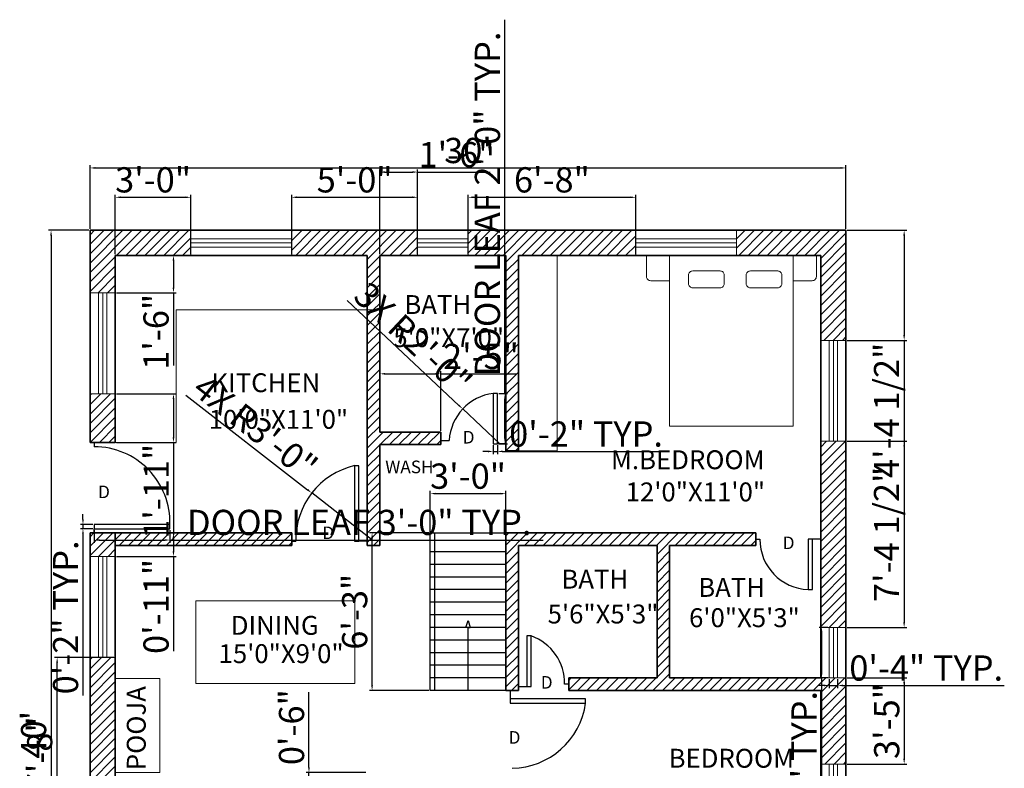
# Model space of a CAD drawing. Units: inches. Extents: x 2105 to 2639, y 1718 to 2373.
# Tile 2 of 2: x 2134 to 2603, y 2017 to 2373. Entities that reach past the tile are written whole.
import ezdxf

# ---------------------------------------------------------------- set-up
doc = ezdxf.new("R2010")
doc.units = ezdxf.units.IN
for name, color, linetype, lineweight in [('A-ANNO-DIMS', 2, 'Continuous', 18), ('A-ANNO-TEXT', 7, 'Continuous', 18), ('A-AREA-IDEN', 7, 'Continuous', 18), ('A-DOOR', 3, 'Continuous', 25), ('A-FLOR-CASE', 9, 'Continuous', 18), ('A-FLOR-STRS', 7, 'Continuous', 25), ('A-FURN', 8, 'Continuous', 18), ('A-GLAZ', 4, 'Continuous', 18), ('A-WALL', 120, 'Continuous', 35), ('A-WALL-PATT', 120, 'Continuous', 13)]:
    doc.layers.add(name, color=color, linetype=linetype, lineweight=lineweight)
doc.styles.get("Standard").update_dxf_attribs({"font": 'arial.ttf'})
doc.dimstyles.new('ISO-25', dxfattribs={"dimtxt": 12, "dimasz": 2.5, "dimexe": 1.25, "dimexo": 0.625, "dimtad": 1, "dimdec": 0, "dimlunit": 3, "dimtxsty": 'Standard', "dimcen": 2.5, "dimadec": 0, "dimazin": 0, "dimtfac": 1, "dimtdec": 0, "dimtmove": 0, "dimatfit": 3, "dimfxl": 1, "dimarcsym": 0})

# ---------------------------------------------------------------- blocks, each defined once
blk = doc.blocks.new('*D1')
at = {"layer": 'A-ANNO-DIMS', "color": 0, "lineweight": -2, "transparency": 16777216}
for p, q in [((2167.87, 2273.92), (2167.87, 2304.21)), ((2170.37, 2302.96), (2525.37, 2302.96)), ((2527.87, 2273.92), (2527.87, 2304.21))]:
    blk.add_line(p, q, dxfattribs=at)
at = {"layer": 'A-ANNO-DIMS', "color": 0, "transparency": 16777216}
for points in [[(2170.37, 2303.38), (2170.37, 2302.54), (2167.87, 2302.96)], [(2525.37, 2303.38), (2525.37, 2302.54), (2527.87, 2302.96)]]:
    blk.add_solid(points, dxfattribs=at)
at = {"layer": 'Defpoints', "color": 0, "transparency": 16777216}
for p in [(2527.87, 2302.96), (2167.87, 2273.29), (2527.87, 2273.29)]:
    blk.add_point(p, dxfattribs=at)
at = {"layer": 'A-ANNO-DIMS', "color": 0, "transparency": 16777216, "insert": (2347.87, 2309.71), "char_height": 12, "attachment_point": 5}
blk.add_mtext("30'", dxfattribs=at)
blk = doc.blocks.new('*D2')
at = {"layer": 'A-ANNO-DIMS', "color": 0, "lineweight": -2, "transparency": 16777216}
for p, q in [((2167.25, 2273.29), (2148.02, 2273.29)), ((2149.27, 2270.79), (2149.27, 1795.79)), ((2167.25, 1793.29), (2148.02, 1793.29))]:
    blk.add_line(p, q, dxfattribs=at)
at = {"layer": 'A-ANNO-DIMS', "color": 0, "transparency": 16777216}
for points in [[(2148.85, 2270.79), (2149.68, 2270.79), (2149.27, 2273.29)], [(2148.85, 1795.79), (2149.68, 1795.79), (2149.27, 1793.29)]]:
    blk.add_solid(points, dxfattribs=at)
at = {"layer": 'Defpoints', "color": 0, "transparency": 16777216}
for p in [(2167.87, 2273.29), (2149.27, 1793.29), (2167.87, 1793.29)]:
    blk.add_point(p, dxfattribs=at)
at = {"layer": 'A-ANNO-DIMS', "color": 0, "transparency": 16777216, "insert": (2142.52, 2033.29), "char_height": 12, "attachment_point": 5, "rotation": 90}
blk.add_mtext("40'", dxfattribs=at)
blk = doc.blocks.new('WIN-GLAZ-48IN')
for p, q in [((0, 4), (48, 4)), ((0, 2), (48, 2)), ((0, 0), (48, 0))]:
    blk.add_line(p, q)
blk = doc.blocks.new('WIN-GLAZ-24IN')
for p, q in [((0, 4), (24, 4)), ((0, 2), (24, 2)), ((0, 0), (24, 0))]:
    blk.add_line(p, q)
blk = doc.blocks.new('DOOR-LEAF-36IN')
for p, q in [((2, 36), (0, 36)), ((0, 36), (0, 0)), ((2, 0), (2, 36)), ((0, 0), (2, 0))]:
    blk.add_line(p, q)
blk = doc.blocks.new('DOOR-LEAF-24IN')
for p, q in [((2, 24), (0, 24)), ((0, 24), (0, 0)), ((2, 0), (2, 24)), ((0, 0), (2, 0))]:
    blk.add_line(p, q)
blk = doc.blocks.new('*D10')
at = {"layer": 'A-ANNO-DIMS', "color": 0, "lineweight": -2, "transparency": 16777216}
for p, q in [((2519.25, 2084.29), (2515.02, 2084.29)), ((2516.27, 2081.79), (2516.27, 2062.79)), ((2519.25, 2060.29), (2515.02, 2060.29)), ((2516.27, 2060.29), (2516.27, 1904.69))]:
    blk.add_line(p, q, dxfattribs=at)
at = {"layer": 'A-ANNO-DIMS', "color": 0, "transparency": 16777216}
for points in [[(2515.86, 2081.79), (2516.69, 2081.79), (2516.27, 2084.29)], [(2515.86, 2062.79), (2516.69, 2062.79), (2516.27, 2060.29)]]:
    blk.add_solid(points, dxfattribs=at)
at = {"layer": 'Defpoints', "color": 0, "transparency": 16777216}
for p in [(2519.87, 2084.29), (2516.27, 2060.29), (2519.87, 2060.29)]:
    blk.add_point(p, dxfattribs=at)
at = {"layer": 'A-ANNO-DIMS', "color": 0, "transparency": 16777216, "insert": (2509.44, 1981.24), "char_height": 12, "attachment_point": 5, "rotation": 90}
blk.add_mtext('WINDOW 2\'-0" TYP.', dxfattribs=at)
blk = doc.blocks.new('*D11')
at = {"layer": 'A-ANNO-DIMS', "color": 0, "lineweight": -2, "transparency": 16777216}
for p, q in [((2519.87, 2059.67), (2519.87, 2055.44)), ((2523.87, 2059.67), (2523.87, 2055.44)), ((2517.37, 2056.69), (2514.87, 2056.69)), ((2519.87, 2056.69), (2523.87, 2056.69)), ((2526.37, 2056.69), (2603.27, 2056.69))]:
    blk.add_line(p, q, dxfattribs=at)
at = {"layer": 'A-ANNO-DIMS', "color": 0, "transparency": 16777216}
for points in [[(2517.37, 2057.11), (2517.37, 2056.28), (2519.87, 2056.69)], [(2526.37, 2057.11), (2526.37, 2056.28), (2523.87, 2056.69)]]:
    blk.add_solid(points, dxfattribs=at)
at = {"layer": 'Defpoints', "color": 0, "transparency": 16777216}
for p in [(2519.87, 2060.29), (2523.87, 2060.29), (2523.87, 2056.69)]:
    blk.add_point(p, dxfattribs=at)
at = {"layer": 'A-ANNO-DIMS', "color": 0, "transparency": 16777216, "insert": (2566.07, 2063.44), "char_height": 12, "attachment_point": 5}
blk.add_mtext('0\'-4" TYP.', dxfattribs=at)
blk = doc.blocks.new('*D12')
at = {"layer": 'A-ANNO-DIMS', "color": 0, "lineweight": -2, "transparency": 16777216}
for p, q in [((2169.87, 2130.67), (2169.87, 2124.64)), ((2205.87, 2130.67), (2205.87, 2124.64)), ((2172.37, 2125.89), (2203.37, 2125.89)), ((2205.87, 2125.89), (2383.71, 2125.89))]:
    blk.add_line(p, q, dxfattribs=at)
at = {"layer": 'A-ANNO-DIMS', "color": 0, "transparency": 16777216}
for points in [[(2172.37, 2126.31), (2172.37, 2125.48), (2169.87, 2125.89)], [(2203.37, 2126.31), (2203.37, 2125.48), (2205.87, 2125.89)]]:
    blk.add_solid(points, dxfattribs=at)
at = {"layer": 'Defpoints', "color": 0, "transparency": 16777216}
for p in [(2169.87, 2131.29), (2205.87, 2131.29), (2205.87, 2125.89)]:
    blk.add_point(p, dxfattribs=at)
at = {"layer": 'A-ANNO-DIMS', "color": 0, "transparency": 16777216, "insert": (2296.04, 2132.73), "char_height": 12, "attachment_point": 5}
blk.add_mtext('DOOR LEAF 3\'-0" TYP.', dxfattribs=at)
blk = doc.blocks.new('*D13')
at = {"layer": 'A-ANNO-DIMS', "color": 0, "lineweight": -2, "transparency": 16777216}
for p, q in [((2164.47, 2135.79), (2164.47, 2138.29)), ((2169.25, 2133.29), (2163.22, 2133.29)), ((2169.25, 2131.29), (2163.22, 2131.29)), ((2164.47, 2133.29), (2164.47, 2131.29)), ((2164.47, 2128.79), (2164.47, 2051.9))]:
    blk.add_line(p, q, dxfattribs=at)
at = {"layer": 'A-ANNO-DIMS', "color": 0, "transparency": 16777216}
for points in [[(2164.06, 2135.79), (2164.89, 2135.79), (2164.47, 2133.29)], [(2164.06, 2128.79), (2164.89, 2128.79), (2164.47, 2131.29)]]:
    blk.add_solid(points, dxfattribs=at)
at = {"layer": 'Defpoints', "color": 0, "transparency": 16777216}
for p in [(2164.47, 2131.29), (2169.87, 2133.29), (2169.87, 2131.29)]:
    blk.add_point(p, dxfattribs=at)
at = {"layer": 'A-ANNO-DIMS', "color": 0, "transparency": 16777216, "insert": (2157.72, 2089.09), "char_height": 12, "attachment_point": 5, "rotation": 90}
blk.add_mtext('0\'-2" TYP.', dxfattribs=at)
blk = doc.blocks.new('*D14')
at = {"layer": 'A-ANNO-DIMS', "color": 0, "lineweight": -2, "transparency": 16777216}
for p, q in [((2365.47, 2195.66), (2365.47, 2373.5)), ((2362.5, 2195.66), (2366.72, 2195.66)), ((2365.47, 2174.16), (2365.47, 2193.16)), ((2362.5, 2171.66), (2366.72, 2171.66))]:
    blk.add_line(p, q, dxfattribs=at)
at = {"layer": 'A-ANNO-DIMS', "color": 0, "transparency": 16777216}
for points in [[(2365.06, 2193.16), (2365.89, 2193.16), (2365.47, 2195.66)], [(2365.06, 2174.16), (2365.89, 2174.16), (2365.47, 2171.66)]]:
    blk.add_solid(points, dxfattribs=at)
at = {"layer": 'Defpoints', "color": 0, "transparency": 16777216}
for p in [(2361.87, 2195.66), (2365.47, 2195.66), (2361.87, 2171.66)]:
    blk.add_point(p, dxfattribs=at)
at = {"layer": 'A-ANNO-DIMS', "color": 0, "transparency": 16777216, "insert": (2358.64, 2285.83), "char_height": 12, "attachment_point": 5, "rotation": 90}
blk.add_mtext('DOOR LEAF 2\'-0" TYP.', dxfattribs=at)
blk = doc.blocks.new('*D15')
at = {"layer": 'A-ANNO-DIMS', "color": 0, "lineweight": -2, "transparency": 16777216}
for p, q in [((2357.37, 2168.06), (2354.87, 2168.06)), ((2359.87, 2171.04), (2359.87, 2166.81)), ((2359.87, 2168.06), (2361.87, 2168.06)), ((2361.87, 2171.04), (2361.87, 2166.81)), ((2364.37, 2168.06), (2441.27, 2168.06))]:
    blk.add_line(p, q, dxfattribs=at)
at = {"layer": 'A-ANNO-DIMS', "color": 0, "transparency": 16777216}
for points in [[(2357.37, 2168.48), (2357.37, 2167.65), (2359.87, 2168.06)], [(2364.37, 2168.48), (2364.37, 2167.65), (2361.87, 2168.06)]]:
    blk.add_solid(points, dxfattribs=at)
at = {"layer": 'Defpoints', "color": 0, "transparency": 16777216}
for p in [(2359.87, 2171.66), (2361.87, 2171.66), (2361.87, 2168.06)]:
    blk.add_point(p, dxfattribs=at)
at = {"layer": 'A-ANNO-DIMS', "color": 0, "transparency": 16777216, "insert": (2404.07, 2174.82), "char_height": 12, "attachment_point": 5}
blk.add_mtext('0\'-2" TYP.', dxfattribs=at)
blk = doc.blocks.new('*D20')
at = {"layer": 'A-ANNO-DIMS', "color": 0, "lineweight": -2, "transparency": 16777216}
for p, q in [((2179.87, 2261.92), (2179.87, 2290.24)), ((2182.37, 2288.99), (2213.37, 2288.99)), ((2215.87, 2261.92), (2215.87, 2290.24))]:
    blk.add_line(p, q, dxfattribs=at)
at = {"layer": 'A-ANNO-DIMS', "color": 0, "transparency": 16777216}
for points in [[(2182.37, 2289.41), (2182.37, 2288.58), (2179.87, 2288.99)], [(2213.37, 2289.41), (2213.37, 2288.58), (2215.87, 2288.99)]]:
    blk.add_solid(points, dxfattribs=at)
at = {"layer": 'Defpoints', "color": 0, "transparency": 16777216}
for p in [(2215.87, 2288.99), (2179.87, 2261.29), (2215.87, 2261.29)]:
    blk.add_point(p, dxfattribs=at)
at = {"layer": 'A-ANNO-DIMS', "color": 0, "transparency": 16777216, "insert": (2197.87, 2295.75), "char_height": 12, "attachment_point": 5}
blk.add_mtext('3\'-0"', dxfattribs=at)
blk = doc.blocks.new('*D21')
at = {"layer": 'A-ANNO-DIMS', "color": 0, "lineweight": -2, "transparency": 16777216}
for p, q in [((2263.87, 2261.92), (2263.87, 2290.24)), ((2266.37, 2288.99), (2321.37, 2288.99)), ((2323.87, 2261.92), (2323.87, 2290.24))]:
    blk.add_line(p, q, dxfattribs=at)
at = {"layer": 'A-ANNO-DIMS', "color": 0, "transparency": 16777216}
for points in [[(2266.37, 2289.41), (2266.37, 2288.58), (2263.87, 2288.99)], [(2321.37, 2289.41), (2321.37, 2288.58), (2323.87, 2288.99)]]:
    blk.add_solid(points, dxfattribs=at)
at = {"layer": 'Defpoints', "color": 0, "transparency": 16777216}
for p in [(2323.87, 2288.99), (2263.87, 2261.29), (2323.87, 2261.29)]:
    blk.add_point(p, dxfattribs=at)
at = {"layer": 'A-ANNO-DIMS', "color": 0, "transparency": 16777216, "insert": (2293.87, 2295.74), "char_height": 12, "attachment_point": 5}
blk.add_mtext('5\'-0"', dxfattribs=at)
blk = doc.blocks.new('*D22')
at = {"layer": 'A-ANNO-DIMS', "color": 0, "lineweight": -2, "transparency": 16777216}
for p, q in [((2347.87, 2261.92), (2347.87, 2290.24)), ((2350.37, 2288.99), (2425.27, 2288.99)), ((2427.77, 2261.92), (2427.77, 2290.24))]:
    blk.add_line(p, q, dxfattribs=at)
at = {"layer": 'A-ANNO-DIMS', "color": 0, "transparency": 16777216}
for points in [[(2350.37, 2289.41), (2350.37, 2288.58), (2347.87, 2288.99)], [(2425.27, 2289.41), (2425.27, 2288.58), (2427.77, 2288.99)]]:
    blk.add_solid(points, dxfattribs=at)
at = {"layer": 'Defpoints', "color": 0, "transparency": 16777216}
for p in [(2427.77, 2288.99), (2347.87, 2261.29), (2427.77, 2261.29)]:
    blk.add_point(p, dxfattribs=at)
at = {"layer": 'A-ANNO-DIMS', "color": 0, "transparency": 16777216, "insert": (2387.82, 2295.74), "char_height": 12, "attachment_point": 5}
blk.add_mtext('6\'-8"', dxfattribs=at)
blk = doc.blocks.new('*D23')
at = {"layer": 'A-ANNO-DIMS', "color": 0, "lineweight": -2, "transparency": 16777216}
for p, q in [((2528.5, 2273.29), (2556.82, 2273.29)), ((2555.57, 2270.79), (2555.57, 2223.42)), ((2528.5, 2220.92), (2556.82, 2220.92)), ((2555.57, 2220.92), (2555.57, 2156.83))]:
    blk.add_line(p, q, dxfattribs=at)
at = {"layer": 'A-ANNO-DIMS', "color": 0, "transparency": 16777216}
for points in [[(2555.16, 2270.79), (2555.99, 2270.79), (2555.57, 2273.29)], [(2555.16, 2223.42), (2555.99, 2223.42), (2555.57, 2220.92)]]:
    blk.add_solid(points, dxfattribs=at)
at = {"layer": 'Defpoints', "color": 0, "transparency": 16777216}
for p in [(2527.87, 2273.29), (2527.87, 2220.92), (2555.57, 2220.92)]:
    blk.add_point(p, dxfattribs=at)
at = {"layer": 'A-ANNO-DIMS', "color": 0, "transparency": 16777216, "insert": (2548.74, 2187.62), "char_height": 12, "attachment_point": 5, "rotation": 90}
blk.add_mtext('4\'-4 1/2"', dxfattribs=at)
blk = doc.blocks.new('*D24')
at = {"layer": 'A-ANNO-DIMS', "color": 0, "lineweight": -2, "transparency": 16777216}
for p, q in [((2528.5, 2172.92), (2556.82, 2172.92)), ((2555.57, 2170.42), (2555.57, 2086.79)), ((2528.5, 2084.29), (2556.82, 2084.29))]:
    blk.add_line(p, q, dxfattribs=at)
at = {"layer": 'A-ANNO-DIMS', "color": 0, "transparency": 16777216}
for points in [[(2555.16, 2170.42), (2555.99, 2170.42), (2555.57, 2172.92)], [(2555.16, 2086.79), (2555.99, 2086.79), (2555.57, 2084.29)]]:
    blk.add_solid(points, dxfattribs=at)
at = {"layer": 'Defpoints', "color": 0, "transparency": 16777216}
for p in [(2527.87, 2172.92), (2527.87, 2084.29), (2555.57, 2084.29)]:
    blk.add_point(p, dxfattribs=at)
at = {"layer": 'A-ANNO-DIMS', "color": 0, "transparency": 16777216, "insert": (2548.74, 2128.61), "char_height": 12, "attachment_point": 5, "rotation": 90}
blk.add_mtext('7\'-4 1/2"', dxfattribs=at)
blk = doc.blocks.new('*D25')
at = {"layer": 'A-ANNO-DIMS', "color": 0, "lineweight": -2, "transparency": 16777216}
for p, q in [((2528.5, 2060.29), (2556.82, 2060.29)), ((2555.57, 2057.79), (2555.57, 2021.81)), ((2528.5, 2019.31), (2556.82, 2019.31))]:
    blk.add_line(p, q, dxfattribs=at)
at = {"layer": 'A-ANNO-DIMS', "color": 0, "transparency": 16777216}
for points in [[(2555.16, 2057.79), (2555.99, 2057.79), (2555.57, 2060.29)], [(2555.16, 2021.81), (2555.99, 2021.81), (2555.57, 2019.31)]]:
    blk.add_solid(points, dxfattribs=at)
at = {"layer": 'Defpoints', "color": 0, "transparency": 16777216}
for p in [(2527.87, 2060.29), (2527.87, 2019.31), (2555.57, 2019.31)]:
    blk.add_point(p, dxfattribs=at)
at = {"layer": 'A-ANNO-DIMS', "color": 0, "transparency": 16777216, "insert": (2548.82, 2039.8), "char_height": 12, "attachment_point": 5, "rotation": 90}
blk.add_mtext('3\'-5"', dxfattribs=at)
blk = doc.blocks.new('*D28')
at = {"layer": 'A-ANNO-DIMS', "color": 0, "lineweight": -2, "transparency": 16777216}
for p, q in [((2180.5, 2261.29), (2208.82, 2261.29)), ((2207.57, 2258.79), (2207.57, 2246.01)), ((2180.5, 2243.51), (2208.82, 2243.51)), ((2207.57, 2243.51), (2207.57, 2208.99))]:
    blk.add_line(p, q, dxfattribs=at)
at = {"layer": 'A-ANNO-DIMS', "color": 0, "transparency": 16777216}
for points in [[(2207.16, 2258.79), (2207.99, 2258.79), (2207.57, 2261.29)], [(2207.16, 2246.01), (2207.99, 2246.01), (2207.57, 2243.51)]]:
    blk.add_solid(points, dxfattribs=at)
at = {"layer": 'Defpoints', "color": 0, "transparency": 16777216}
for p in [(2179.87, 2261.29), (2179.87, 2243.51), (2207.57, 2243.51)]:
    blk.add_point(p, dxfattribs=at)
at = {"layer": 'A-ANNO-DIMS', "color": 0, "transparency": 16777216, "insert": (2200.82, 2225), "char_height": 12, "attachment_point": 5, "rotation": 90}
blk.add_mtext('1\'-6"', dxfattribs=at)
blk = doc.blocks.new('*D29')
at = {"layer": 'A-ANNO-DIMS', "color": 0, "lineweight": -2, "transparency": 16777216}
for p, q in [((2180.5, 2195.51), (2208.82, 2195.51)), ((2207.57, 2193.01), (2207.57, 2174.79)), ((2180.5, 2172.29), (2208.82, 2172.29)), ((2207.57, 2172.29), (2207.57, 2128.45))]:
    blk.add_line(p, q, dxfattribs=at)
at = {"layer": 'A-ANNO-DIMS', "color": 0, "transparency": 16777216}
for points in [[(2207.16, 2193.01), (2207.99, 2193.01), (2207.57, 2195.51)], [(2207.16, 2174.79), (2207.99, 2174.79), (2207.57, 2172.29)]]:
    blk.add_solid(points, dxfattribs=at)
at = {"layer": 'Defpoints', "color": 0, "transparency": 16777216}
for p in [(2179.87, 2195.51), (2179.87, 2172.29), (2207.57, 2172.29)]:
    blk.add_point(p, dxfattribs=at)
at = {"layer": 'A-ANNO-DIMS', "color": 0, "transparency": 16777216, "insert": (2200.92, 2149.12), "char_height": 12, "attachment_point": 5, "rotation": 90}
blk.add_mtext('1\'-11"', dxfattribs=at)
blk = doc.blocks.new('*D30')
at = {"layer": 'A-ANNO-DIMS', "color": 0, "lineweight": -2, "transparency": 16777216}
for p, q in [((2180.5, 2129.29), (2208.82, 2129.29)), ((2207.57, 2126.79), (2207.57, 2120.56)), ((2180.5, 2118.06), (2208.82, 2118.06)), ((2207.57, 2118.06), (2207.57, 2073.09))]:
    blk.add_line(p, q, dxfattribs=at)
at = {"layer": 'A-ANNO-DIMS', "color": 0, "transparency": 16777216}
for points in [[(2207.16, 2126.79), (2207.99, 2126.79), (2207.57, 2129.29)], [(2207.16, 2120.56), (2207.99, 2120.56), (2207.57, 2118.06)]]:
    blk.add_solid(points, dxfattribs=at)
at = {"layer": 'Defpoints', "color": 0, "transparency": 16777216}
for p in [(2179.87, 2129.29), (2179.87, 2118.06), (2207.57, 2118.06)]:
    blk.add_point(p, dxfattribs=at)
at = {"layer": 'A-ANNO-DIMS', "color": 0, "transparency": 16777216, "insert": (2200.82, 2094.32), "char_height": 12, "attachment_point": 5, "rotation": 90}
blk.add_mtext('0\'-11"', dxfattribs=at)
blk = doc.blocks.new('*D31')
at = {"layer": 'A-ANNO-DIMS', "color": 0, "lineweight": -2, "transparency": 16777216}
for p, q in [((2179.25, 2070.06), (2150.92, 2070.06)), ((2152.17, 1980.35), (2152.17, 2067.56)), ((2179.25, 1977.85), (2150.92, 1977.85))]:
    blk.add_line(p, q, dxfattribs=at)
at = {"layer": 'A-ANNO-DIMS', "color": 0, "transparency": 16777216}
for points in [[(2151.76, 2067.56), (2152.59, 2067.56), (2152.17, 2070.06)], [(2151.76, 1980.35), (2152.59, 1980.35), (2152.17, 1977.85)]]:
    blk.add_solid(points, dxfattribs=at)
at = {"layer": 'Defpoints', "color": 0, "transparency": 16777216}
for p in [(2152.17, 2070.06), (2179.87, 2070.06), (2179.87, 1977.85)]:
    blk.add_point(p, dxfattribs=at)
at = {"layer": 'A-ANNO-DIMS', "color": 0, "transparency": 16777216, "insert": (2145.42, 2023.95), "char_height": 12, "attachment_point": 5, "rotation": 90}
blk.add_mtext('7\'-8"', dxfattribs=at)
blk = doc.blocks.new('*D35')
at = {"layer": 'A-ANNO-DIMS', "color": 0, "lineweight": -2, "transparency": 16777216}
for p, q in [((2329.87, 2120.92), (2329.87, 2149.24)), ((2332.37, 2147.99), (2363.37, 2147.99)), ((2365.87, 2120.92), (2365.87, 2149.24))]:
    blk.add_line(p, q, dxfattribs=at)
at = {"layer": 'A-ANNO-DIMS', "color": 0, "transparency": 16777216}
for points in [[(2332.37, 2148.41), (2332.37, 2147.58), (2329.87, 2147.99)], [(2363.37, 2148.41), (2363.37, 2147.58), (2365.87, 2147.99)]]:
    blk.add_solid(points, dxfattribs=at)
at = {"layer": 'Defpoints', "color": 0, "transparency": 16777216}
for p in [(2365.87, 2147.99), (2329.87, 2120.29), (2365.87, 2120.29)]:
    blk.add_point(p, dxfattribs=at)
at = {"layer": 'A-ANNO-DIMS', "color": 0, "transparency": 16777216, "insert": (2347.87, 2154.75), "char_height": 12, "attachment_point": 5}
blk.add_mtext('3\'-0"', dxfattribs=at)
blk = doc.blocks.new('*D36')
at = {"layer": 'A-ANNO-DIMS', "color": 0, "lineweight": -2, "transparency": 16777216}
for p, q in [((2329.25, 2129.29), (2300.92, 2129.29)), ((2302.17, 2056.79), (2302.17, 2126.79)), ((2329.25, 2054.29), (2300.92, 2054.29))]:
    blk.add_line(p, q, dxfattribs=at)
at = {"layer": 'A-ANNO-DIMS', "color": 0, "transparency": 16777216}
for points in [[(2301.76, 2126.79), (2302.59, 2126.79), (2302.17, 2129.29)], [(2301.76, 2056.79), (2302.59, 2056.79), (2302.17, 2054.29)]]:
    blk.add_solid(points, dxfattribs=at)
at = {"layer": 'Defpoints', "color": 0, "transparency": 16777216}
for p in [(2302.17, 2129.29), (2329.87, 2129.29), (2329.87, 2054.29)]:
    blk.add_point(p, dxfattribs=at)
at = {"layer": 'A-ANNO-DIMS', "color": 0, "transparency": 16777216, "insert": (2295.42, 2091.79), "char_height": 12, "attachment_point": 5, "rotation": 90}
blk.add_mtext('6\'-3"', dxfattribs=at)
blk = doc.blocks.new('*D38')
at = {"layer": 'A-ANNO-DIMS', "color": 0, "lineweight": -2, "transparency": 16777216}
for p, q in [((2272.1, 2017.79), (2272.1, 2053.44)), ((2299.18, 2015.29), (2270.85, 2015.29)), ((2272.1, 2009.29), (2272.1, 2015.29)), ((2299.18, 2009.29), (2270.85, 2009.29)), ((2272.1, 2006.79), (2272.1, 2004.29))]:
    blk.add_line(p, q, dxfattribs=at)
at = {"layer": 'A-ANNO-DIMS', "color": 0, "transparency": 16777216}
for points in [[(2271.69, 2017.79), (2272.52, 2017.79), (2272.1, 2015.29)], [(2271.69, 2006.79), (2272.52, 2006.79), (2272.1, 2009.29)]]:
    blk.add_solid(points, dxfattribs=at)
at = {"layer": 'Defpoints', "color": 0, "transparency": 16777216}
for p in [(2272.1, 2015.29), (2299.8, 2015.29), (2299.8, 2009.29)]:
    blk.add_point(p, dxfattribs=at)
at = {"layer": 'A-ANNO-DIMS', "color": 0, "transparency": 16777216, "insert": (2265.35, 2036.87), "char_height": 12, "attachment_point": 5, "rotation": 90}
blk.add_mtext('0\'-6"', dxfattribs=at)
blk = doc.blocks.new('*D39')
at = {"layer": 'A-ANNO-DIMS', "color": 0, "lineweight": -2, "transparency": 16777216}
for p, q in [((2305.87, 2177.92), (2305.87, 2206.24)), ((2308.37, 2204.99), (2332.37, 2204.99)), ((2334.87, 2177.92), (2334.87, 2206.24)), ((2334.87, 2204.99), (2370.73, 2204.99))]:
    blk.add_line(p, q, dxfattribs=at)
at = {"layer": 'A-ANNO-DIMS', "color": 0, "transparency": 16777216}
for points in [[(2308.37, 2205.41), (2308.37, 2204.58), (2305.87, 2204.99)], [(2332.37, 2205.41), (2332.37, 2204.58), (2334.87, 2204.99)]]:
    blk.add_solid(points, dxfattribs=at)
at = {"layer": 'Defpoints', "color": 0, "transparency": 16777216}
for p in [(2334.87, 2204.99), (2305.87, 2177.29), (2334.87, 2177.29)]:
    blk.add_point(p, dxfattribs=at)
at = {"layer": 'A-ANNO-DIMS', "color": 0, "transparency": 16777216, "insert": (2354.05, 2211.74), "char_height": 12, "attachment_point": 5}
blk.add_mtext('2\'-5"', dxfattribs=at)
blk = doc.blocks.new('*D40')
at = {"layer": 'A-ANNO-DIMS', "color": 0, "lineweight": -2, "transparency": 16777216}
for p, q in [((2305.87, 2261.92), (2305.87, 2302.24)), ((2308.37, 2300.99), (2321.37, 2300.99)), ((2323.87, 2261.92), (2323.87, 2302.24)), ((2323.87, 2300.99), (2358.39, 2300.99))]:
    blk.add_line(p, q, dxfattribs=at)
at = {"layer": 'A-ANNO-DIMS', "color": 0, "transparency": 16777216}
for points in [[(2308.37, 2301.41), (2308.37, 2300.58), (2305.87, 2300.99)], [(2321.37, 2301.41), (2321.37, 2300.58), (2323.87, 2300.99)]]:
    blk.add_solid(points, dxfattribs=at)
at = {"layer": 'Defpoints', "color": 0, "transparency": 16777216}
for p in [(2323.87, 2300.99), (2305.87, 2261.29), (2323.87, 2261.29)]:
    blk.add_point(p, dxfattribs=at)
at = {"layer": 'A-ANNO-DIMS', "color": 0, "transparency": 16777216, "insert": (2342.38, 2307.74), "char_height": 12, "attachment_point": 5}
blk.add_mtext('1\'-6"', dxfattribs=at)
blk = doc.blocks.new('*D42')
at = {"layer": 'A-ANNO-DIMS', "color": 0, "lineweight": -2, "transparency": 16777216}
for p, q in [((2213.53, 2194.89), (2271.47, 2149.83)), ((2301.86, 2126.19), (2273.45, 2148.29))]:
    blk.add_line(p, q, dxfattribs=at)
at = {"layer": 'A-ANNO-DIMS', "color": 0, "transparency": 16777216}
blk.add_solid([(2271.73, 2150.15), (2271.22, 2149.5), (2273.45, 2148.29)], dxfattribs=at)
at = {"layer": 'Defpoints', "color": 0, "transparency": 16777216}
for p in [(2273.45, 2148.29), (2301.86, 2126.19)]:
    blk.add_point(p, dxfattribs=at)
at = {"layer": 'A-ANNO-DIMS', "color": 0, "transparency": 16777216, "insert": (2245.66, 2178.46), "char_height": 12, "attachment_point": 5, "rotation": 322.1257}
blk.add_mtext('4X R3\'-0"', dxfattribs=at)
blk = doc.blocks.new('*D43')
at = {"layer": 'A-ANNO-DIMS', "color": 0, "lineweight": -2, "transparency": 16777216}
for p, q in [((2290.35, 2239.88), (2343.51, 2189.98)), ((2362.83, 2171.85), (2345.33, 2188.27))]:
    blk.add_line(p, q, dxfattribs=at)
at = {"layer": 'A-ANNO-DIMS', "color": 0, "transparency": 16777216}
blk.add_solid([(2343.79, 2190.29), (2343.22, 2189.68), (2345.33, 2188.27)], dxfattribs=at)
at = {"layer": 'Defpoints', "color": 0, "transparency": 16777216}
for p in [(2345.33, 2188.27), (2362.83, 2171.85)]:
    blk.add_point(p, dxfattribs=at)
at = {"layer": 'A-ANNO-DIMS', "color": 0, "transparency": 16777216, "insert": (2320.64, 2220.71), "char_height": 12, "attachment_point": 5, "rotation": 316.8117}
blk.add_mtext('3X R2\'-0"', dxfattribs=at)

msp = doc.modelspace()

# ---------------------------------------------------------------- hatches: boundary and pattern name
at = {"layer": 'A-WALL-PATT'}
h = msp.add_hatch(dxfattribs=at)
h.set_pattern_fill('ANSI31', color=256)
h.paths.add_polyline_path([(2215.87, 2273.29), (2167.87, 2273.29), (2167.87, 2243.51), (2179.87, 2243.51), (2179.87, 2261.29), (2215.87, 2261.29)])
h = msp.add_hatch(dxfattribs=at)
h.set_pattern_fill('ANSI31', color=256)
h.paths.add_polyline_path([(2323.87, 2273.29), (2263.87, 2273.29), (2263.87, 2261.29), (2299.87, 2261.29), (2299.87, 2235.4), (2305.87, 2235.4), (2305.87, 2261.29), (2323.87, 2261.29)])
h = msp.add_hatch(dxfattribs=at)
h.set_pattern_fill('ANSI31', color=256)
h.paths.add_polyline_path([(2427.77, 2273.29), (2347.87, 2273.29), (2347.87, 2261.29), (2365.87, 2261.29), (2365.87, 2168.36), (2371.87, 2168.36), (2371.87, 2261.29), (2427.77, 2261.29)])
h = msp.add_hatch(dxfattribs=at)
h.set_pattern_fill('ANSI31', color=256)
h.paths.add_polyline_path([(2527.87, 2273.29), (2475.77, 2273.29), (2475.77, 2261.29), (2502.75, 2261.29), (2515.87, 2261.29), (2515.87, 2220.92), (2527.87, 2220.92)])
h = msp.add_hatch(dxfattribs=at)
h.set_pattern_fill('ANSI31', color=256)
h.paths.add_polyline_path([(2305.87, 2235.4), (2299.87, 2235.4), (2299.87, 2129.29), (2299.87, 2123.29), (2305.87, 2123.29), (2305.87, 2171.29), (2334.87, 2171.29), (2334.87, 2173.29), (2334.87, 2177.29), (2305.87, 2177.29)])
h = msp.add_hatch(dxfattribs=at)
h.set_pattern_fill('ANSI31', color=256)
h.paths.add_polyline_path([(2179.87, 2195.51), (2167.87, 2195.51), (2167.87, 2172.29), (2169.87, 2172.29), (2179.87, 2172.29)])
h = msp.add_hatch(dxfattribs=at)
h.set_pattern_fill('ANSI31', color=256)
h.paths.add_polyline_path([(2527.87, 2172.92), (2515.87, 2172.92), (2515.87, 2084.29), (2527.87, 2084.29)])
h = msp.add_hatch(dxfattribs=at)
h.set_pattern_fill('ANSI31', color=256)
h.paths.add_polyline_path([(2179.87, 2129.29), (2167.87, 2129.29), (2167.87, 2118.06), (2179.87, 2118.06)])
h = msp.add_hatch(dxfattribs=at)
h.set_pattern_fill('ANSI31', color=256)
h.paths.add_polyline_path([(2263.87, 2129.29), (2179.87, 2129.29), (2179.87, 2123.29), (2263.87, 2123.29), (2263.87, 2125.29)])
h = msp.add_hatch(dxfattribs=at)
h.set_pattern_fill('ANSI31', color=256)
h.paths.add_polyline_path([(2527.87, 2060.29), (2515.87, 2060.29), (2443.87, 2060.29), (2443.87, 2123.29), (2484.87, 2123.29), (2484.87, 2129.29), (2365.87, 2129.29), (2365.87, 2054.29), (2367.87, 2054.29), (2371.87, 2054.29), (2371.87, 2056.29), (2371.87, 2123.29), (2437.87, 2123.29), (2437.87, 2060.29), (2395.87, 2060.29), (2395.87, 2054.29), (2515.87, 2054.29), (2515.87, 2019.31), (2527.87, 2019.31)])
h = msp.add_hatch(dxfattribs=at)
h.set_pattern_fill('ANSI31', color=256)
h.paths.add_polyline_path([(2179.87, 2070.06), (2167.87, 2070.06), (2167.87, 1977.85), (2179.87, 1977.85)])

# ---------------------------------------------------------------- linework, layer by layer
at = {"layer": 'A-DOOR'}
for p, q in [((2167.87, 2172.29), (2169.87, 2172.29)), ((2169.87, 2172.29), (2169.87, 2170.29)), ((2334.87, 2171.29), (2334.87, 2173.29)), ((2334.87, 2173.29), (2338.87, 2173.29)), ((2365.87, 2171.66), (2361.87, 2171.66)), ((2365.87, 2168.36), (2365.87, 2171.66)), ((2167.87, 2129.29), (2169.87, 2129.29)), ((2169.87, 2129.29), (2169.87, 2131.29)), ((2484.87, 2129.29), (2484.87, 2126.29)), ((2515.87, 2129.29), (2515.87, 2126.29)), ((2263.87, 2123.29), (2263.87, 2125.29)), ((2263.87, 2125.29), (2265.87, 2125.29)), ((2299.87, 2125.29), (2295.87, 2125.29)), ((2299.87, 2123.29), (2299.87, 2125.29)), ((2484.87, 2126.29), (2486.87, 2126.29)), ((2515.87, 2126.29), (2511.87, 2126.29)), ((2365.87, 2054.29), (2367.87, 2054.29)), ((2367.87, 2054.29), (2367.87, 2050.29)), ((2371.87, 2054.29), (2371.87, 2056.29)), ((2371.87, 2056.29), (2375.87, 2056.29)), ((2395.87, 2057.29), (2393.87, 2057.29)), ((2395.87, 2054.29), (2395.87, 2057.29))]:
    msp.add_line(p, q, dxfattribs=at)
for centre, radius, start, end in [((2362.83, 2171.85), 24, 97.0761, 176.5494), ((2169.89, 2134.29), 36, 358.4082, 90.0221), ((2301.86, 2126.19), 36, 102.8213, 181.4287), ((2510.87, 2126.27), 24, 179.9502, 267.612), ((2369.88, 2057.66), 24, 359.1129, 70.5361), ((2368.22, 2053.29), 36, 271.0376, 352.0259)]:
    msp.add_arc(centre, radius, start, end, dxfattribs=at)
at = {"layer": 'A-FLOR-CASE'}
for p, q in [((2390.24, 2168.36), (2390.24, 2261.29)), ((2208.82, 2172.29), (2208.82, 2235.4)), ((2208.82, 2235.4), (2305.87, 2235.4)), ((2179.87, 2172.29), (2208.82, 2172.29)), ((2371.87, 2168.36), (2390.24, 2168.36))]:
    msp.add_line(p, q, dxfattribs=at)
msp.add_lwpolyline([(2179.87, 2015.29), (2201.1, 2015.29), (2201.1, 2060.06), (2179.87, 2060.06)], close=True, dxfattribs=at)
at = {"layer": 'A-FLOR-STRS'}
for p, q in [((2329.87, 2054.29), (2329.87, 2129.29)), ((2329.87, 2129.29), (2365.87, 2129.29)), ((2329.87, 2129.29), (2331.87, 2129.29)), ((2331.87, 2129.29), (2331.87, 2054.29)), ((2365.87, 2120.29), (2329.87, 2120.29)), ((2365.87, 2120.29), (2329.87, 2120.29)), ((2365.87, 2114.29), (2329.87, 2114.29)), ((2365.87, 2108.29), (2329.87, 2108.29)), ((2365.87, 2102.29), (2329.87, 2102.29)), ((2365.87, 2096.29), (2329.87, 2096.29)), ((2365.87, 2090.29), (2329.87, 2090.29)), ((2346.87, 2084.29), (2347.87, 2087.56)), ((2347.87, 2087.56), (2348.87, 2084.29)), ((2365.87, 2084.29), (2329.87, 2084.29)), ((2347.87, 2084.29), (2346.87, 2084.29)), ((2347.87, 2054.29), (2347.87, 2084.29)), ((2347.87, 2084.29), (2348.87, 2084.29)), ((2365.87, 2078.29), (2329.87, 2078.29)), ((2365.87, 2072.29), (2329.87, 2072.29)), ((2365.87, 2066.29), (2329.87, 2066.29)), ((2365.87, 2060.29), (2329.87, 2060.29)), ((2365.87, 2054.29), (2329.87, 2054.29))]:
    msp.add_line(p, q, dxfattribs=at)
at = {"layer": 'A-FURN'}
for points in [[(2443.87, 2261.29), (2432.87, 2261.29), (2432.87, 2251.29, 0.414214), (2434.87, 2249.29), (2443.87, 2249.29)], [(2502.75, 2261.29), (2513.75, 2261.29), (2513.75, 2251.29, -0.414214), (2511.75, 2249.29), (2502.75, 2249.29)], [(2454.89, 2253.95), (2467.89, 2253.95, -0.414214), (2469.89, 2251.95), (2469.89, 2247.95, -0.414214), (2467.89, 2245.95), (2454.89, 2245.95, -0.414214), (2452.89, 2247.95), (2452.89, 2251.95, -0.414214)], [(2482.33, 2253.95), (2495.33, 2253.95, -0.414214), (2497.33, 2251.95), (2497.33, 2247.95, -0.414214), (2495.33, 2245.95), (2482.33, 2245.95, -0.414214), (2480.33, 2247.95), (2480.33, 2251.95, -0.414214)]]:
    msp.add_lwpolyline(points, format="xyb", close=True, dxfattribs=at)
for points in [[(2443.87, 2261.29), (2502.75, 2261.29), (2502.75, 2180.11), (2443.87, 2180.11)], [(2218.16, 2097), (2294.01, 2097), (2294.01, 2057.69), (2218.16, 2057.69)]]:
    msp.add_lwpolyline(points, close=True, dxfattribs=at)
at = {"layer": 'A-GLAZ'}
for p, q in [((2215.87, 2261.29), (2215.87, 2273.29)), ((2263.87, 2261.29), (2263.87, 2273.29)), ((2323.87, 2261.29), (2323.87, 2273.29)), ((2347.87, 2261.29), (2347.87, 2273.29)), ((2427.77, 2261.29), (2427.77, 2273.29)), ((2475.77, 2261.29), (2475.77, 2273.29)), ((2167.87, 2243.51), (2179.87, 2243.51)), ((2527.87, 2220.92), (2515.87, 2220.92)), ((2167.87, 2195.51), (2179.87, 2195.51)), ((2527.87, 2172.92), (2515.87, 2172.92)), ((2167.87, 2118.06), (2179.87, 2118.06)), ((2527.87, 2084.29), (2515.87, 2084.29)), ((2167.87, 2070.06), (2179.87, 2070.06)), ((2527.87, 2060.29), (2515.87, 2060.29)), ((2527.87, 2019.31), (2515.87, 2019.31))]:
    msp.add_line(p, q, dxfattribs=at)
at = {"layer": 'A-WALL'}
for p, q in [((2179.87, 2261.29), (2299.87, 2261.29)), ((2179.87, 2172.29), (2179.87, 2261.29)), ((2299.87, 2129.29), (2299.87, 2261.29)), ((2305.87, 2177.29), (2305.87, 2261.29)), ((2305.87, 2261.29), (2365.87, 2261.29)), ((2365.87, 2168.36), (2365.87, 2261.29)), ((2371.87, 2168.36), (2371.87, 2261.29)), ((2371.87, 2261.29), (2515.87, 2261.29)), ((2515.87, 2261.29), (2515.87, 2060.29)), ((2305.87, 2177.29), (2334.87, 2177.29)), ((2334.87, 2171.29), (2334.87, 2177.29)), ((2179.87, 2172.29), (2167.87, 2172.29)), ((2305.87, 2123.29), (2305.87, 2171.29)), ((2305.87, 2171.29), (2334.87, 2171.29)), ((2365.87, 2168.36), (2371.87, 2168.36)), ((2179.87, 2129.29), (2167.87, 2129.29)), ((2179.87, 1865.29), (2179.87, 2129.29)), ((2179.87, 2129.29), (2263.87, 2129.29)), ((2263.87, 2129.29), (2263.87, 2123.29)), ((2299.87, 2129.29), (2299.87, 2123.29)), ((2365.87, 2129.29), (2484.87, 2129.29)), ((2365.87, 2054.29), (2365.87, 2129.29)), ((2484.87, 2129.29), (2484.87, 2123.29)), ((2515.87, 2129.29), (2515.87, 2123.29)), ((2179.87, 2123.29), (2263.87, 2123.29)), ((2299.87, 2123.29), (2305.87, 2123.29)), ((2371.87, 2123.29), (2437.87, 2123.29)), ((2371.87, 2054.29), (2371.87, 2123.29)), ((2437.87, 2060.29), (2437.87, 2123.29)), ((2443.87, 2060.29), (2443.87, 2123.29)), ((2443.87, 2123.29), (2484.87, 2123.29)), ((2395.87, 2060.29), (2437.87, 2060.29)), ((2395.87, 2054.29), (2395.87, 2060.29)), ((2443.87, 2060.29), (2515.87, 2060.29)), ((2365.87, 2054.29), (2371.87, 2054.29)), ((2395.87, 2054.29), (2515.87, 2054.29)), ((2515.87, 2054.29), (2515.87, 1931.29))]:
    msp.add_line(p, q, dxfattribs=at)
msp.add_lwpolyline([(2167.87, 2172.29), (2167.87, 2273.29), (2527.87, 2273.29), (2527.87, 1793.29), (2167.87, 1793.29), (2167.87, 2129.29)], dxfattribs=at)

# ---------------------------------------------------------------- block references
at = {"layer": 'A-DOOR'}
for name, p in [('DOOR-LEAF-24IN', (2359.87, 2171.66)), ('DOOR-LEAF-36IN', (2293.87, 2125.29)), ('DOOR-LEAF-24IN', (2509.87, 2102.29))]:
    msp.add_blockref(name, p, dxfattribs=at)
for name, p, rotation in [('DOOR-LEAF-36IN', (2169.87, 2133.29), 269.9999999999942), ('DOOR-LEAF-24IN', (2377.87, 2080.29), 180), ('DOOR-LEAF-36IN', (2403.87, 2048.29), 89.99999999999714)]:
    msp.add_blockref(name, p, dxfattribs=dict(at, rotation=rotation))
at = {"layer": 'A-GLAZ'}
for name, p in [('WIN-GLAZ-48IN', (2215.87, 2265.29)), ('WIN-GLAZ-24IN', (2323.87, 2265.29))]:
    msp.add_blockref(name, p, dxfattribs=at)
for name, p, rotation in [('WIN-GLAZ-48IN', (2475.77, 2269.29), 180), ('WIN-GLAZ-48IN', (2175.87, 2195.51), 90.00000000000097), ('WIN-GLAZ-48IN', (2519.87, 2220.92), 270.0000000000021), ('WIN-GLAZ-48IN', (2175.87, 2070.06), 90.00000000000205), ('WIN-GLAZ-24IN', (2519.87, 2084.29), 269.9999999999961), ('WIN-GLAZ-48IN', (2519.87, 2019.31), 270.0000000000023)]:
    msp.add_blockref(name, p, dxfattribs=dict(at, rotation=rotation))

# ---------------------------------------------------------------- texts
at = {"layer": 'A-ANNO-TEXT'}
for p in [(2345.34, 2171.83), (2171.67, 2145.83), (2278.51, 2126.34), (2497.73, 2121.57), (2382.52, 2055.18), (2367.2, 2028.98)]:
    msp.add_attdef('D', p, '', height=6, dxfattribs=at)
at = {"layer": 'A-AREA-IDEN'}
for tag, p, height in [('BATH', (2317.54, 2233.45), 9), ('5\'0"X7\'0"', (2312.29, 2217.72), 9), ('KITCHEN', (2225.7, 2196.26), 9), ('10\'0"X11\'0"', (2224.38, 2178.83), 9), ('M.BEDROOM', (2415.95, 2159.6), 9), ('WASH', (2308.44, 2157.71), 6), ('12\'0"X11\'0"', (2422.94, 2144.3), 9), ('BATH', (2392.33, 2102.79), 9), ('BATH', (2457.5, 2098.86), 9), ('5\'6"X5\'3"', (2385.77, 2086.19), 9), ('6\'0"X5\'3"', (2453.12, 2084.44), 9), ('DINING', (2234.88, 2080.81), 9), ('15\'0"X9\'0"', (2229.05, 2067.34), 9), ('BEDROOM', (2443.39, 2017.56), 9)]:
    msp.add_attdef(tag, p, '', height=height, dxfattribs=at)
msp.add_attdef('POOJA', (2194.36, 2016.39), '', height=9, rotation=90, dxfattribs=at)

# ---------------------------------------------------------------- dimensions: what is measured, and where the dimension line sits
at = {"layer": 'A-ANNO-DIMS'}
for base, p1, p2, angle, text, picture, middle in [((2365.47, 2195.66), (2361.87, 2171.66), (2361.87, 2195.66), 90, 'DOOR LEAF <> TYP.', '*D14', (2358.64, 2285.83)), ((2164.47, 2131.29), (2169.87, 2133.29), (2169.87, 2131.29), 270, '<> TYP.', '*D13', (2157.72, 2089.09)), ((2516.27, 2060.29), (2519.87, 2084.29), (2519.87, 2060.29), 270, 'WINDOW <> TYP.', '*D10', (2509.44, 1981.24))]:
    dim = msp.add_linear_dim(base=base, p1=p1, p2=p2, angle=angle, text=text, dimstyle='ISO-25', override={"dimdec": 1, "dimlfac": 1, "dimrnd": 0, "dimzin": 1, "dimdsep": 46, "dimlunit": 4, "dimfrac": 2}, dxfattribs=at)
    dim.commit()
    dim.dimension.update_dxf_attribs({"geometry": picture, "text_midpoint": middle})
for base, p1, p2, override, picture, middle in [((2527.87, 2302.96), (2167.87, 2273.29), (2527.87, 2273.29), {"dimclrd": 0, "dimclre": 0, "dimclrt": 0}, '*D1', (2347.87, 2309.71)), ((2323.87, 2300.99), (2305.87, 2261.29), (2323.87, 2261.29), {"dimdec": 1, "dimlfac": 1, "dimrnd": 0, "dimzin": 1, "dimdsep": 46, "dimlunit": 4, "dimfrac": 2}, '*D40', (2342.38, 2307.74)), ((2215.87, 2288.99), (2179.87, 2261.29), (2215.87, 2261.29), {"dimdec": 1, "dimlfac": 1, "dimrnd": 0, "dimzin": 1, "dimdsep": 46, "dimlunit": 4, "dimfrac": 2}, '*D20', (2197.87, 2295.75)), ((2323.87, 2288.99), (2263.87, 2261.29), (2323.87, 2261.29), {"dimdec": 1, "dimlfac": 1, "dimrnd": 0, "dimzin": 1, "dimdsep": 46, "dimlunit": 4, "dimfrac": 2}, '*D21', (2293.87, 2295.74)), ((2427.77, 2288.99), (2347.87, 2261.29), (2427.77, 2261.29), {"dimdec": 1, "dimlfac": 1, "dimrnd": 0, "dimzin": 1, "dimdsep": 46, "dimlunit": 4, "dimfrac": 2}, '*D22', (2387.82, 2295.74)), ((2334.87, 2204.99), (2305.87, 2177.29), (2334.87, 2177.29), {"dimdec": 1, "dimlfac": 1, "dimrnd": 0, "dimzin": 1, "dimdsep": 46, "dimlunit": 4, "dimfrac": 2}, '*D39', (2354.05, 2211.74)), ((2365.87, 2147.99), (2329.87, 2120.29), (2365.87, 2120.29), {"dimdec": 1, "dimlfac": 1, "dimrnd": 0, "dimzin": 1, "dimdsep": 46, "dimlunit": 4, "dimfrac": 2}, '*D35', (2347.87, 2154.75))]:
    dim = msp.add_linear_dim(base=base, p1=p1, p2=p2, dimstyle='ISO-25', override=override, dxfattribs=at)
    dim.commit()
    dim.dimension.update_dxf_attribs({"geometry": picture, "text_midpoint": middle})
for base, p1, p2, angle, override, picture, middle in [((2149.27, 1793.29), (2167.87, 2273.29), (2167.87, 1793.29), 90, {"dimclrd": 0, "dimclre": 0, "dimclrt": 0}, '*D2', (2142.52, 2033.29)), ((2555.57, 2220.92), (2527.87, 2273.29), (2527.87, 2220.92), 90, {"dimdec": 1, "dimlfac": 1, "dimrnd": 0, "dimzin": 1, "dimdsep": 46, "dimlunit": 4, "dimfrac": 2}, '*D23', (2548.74, 2187.62)), ((2207.57, 2243.51), (2179.87, 2261.29), (2179.87, 2243.51), 270, {"dimdec": 1, "dimlfac": 1, "dimrnd": 0, "dimzin": 1, "dimdsep": 46, "dimlunit": 4, "dimfrac": 2}, '*D28', (2200.82, 2225)), ((2207.57, 2172.29), (2179.87, 2195.51), (2179.87, 2172.29), 270, {"dimdec": 1, "dimlfac": 1, "dimrnd": 0, "dimzin": 1, "dimdsep": 46, "dimlunit": 4, "dimfrac": 2}, '*D29', (2200.92, 2149.12)), ((2555.57, 2084.29), (2527.87, 2172.92), (2527.87, 2084.29), 90, {"dimdec": 1, "dimlfac": 1, "dimrnd": 0, "dimzin": 1, "dimdsep": 46, "dimlunit": 4, "dimfrac": 2}, '*D24', (2548.74, 2128.61)), ((2207.57, 2118.06), (2179.87, 2129.29), (2179.87, 2118.06), 270, {"dimdec": 1, "dimlfac": 1, "dimrnd": 0, "dimzin": 1, "dimdsep": 46, "dimlunit": 4, "dimfrac": 2}, '*D30', (2200.82, 2094.32)), ((2302.17, 2129.29), (2329.87, 2054.29), (2329.87, 2129.29), 90, {"dimdec": 1, "dimlfac": 1, "dimrnd": 0, "dimzin": 1, "dimdsep": 46, "dimlunit": 4, "dimfrac": 2}, '*D36', (2295.42, 2091.79)), ((2152.17, 2070.06), (2179.87, 1977.85), (2179.87, 2070.06), 90, {"dimdec": 1, "dimlfac": 1, "dimrnd": 0, "dimzin": 1, "dimdsep": 46, "dimlunit": 4, "dimfrac": 2}, '*D31', (2145.42, 2023.95)), ((2555.57, 2019.31), (2527.87, 2060.29), (2527.87, 2019.31), 90, {"dimdec": 1, "dimlfac": 1, "dimrnd": 0, "dimzin": 1, "dimdsep": 46, "dimlunit": 4, "dimfrac": 2}, '*D25', (2548.82, 2039.8)), ((2272.1, 2015.29), (2299.8, 2009.29), (2299.8, 2015.29), 90, {"dimdec": 1, "dimlfac": 1, "dimrnd": 0, "dimzin": 1, "dimdsep": 46, "dimlunit": 4, "dimfrac": 2}, '*D38', (2265.35, 2036.87))]:
    dim = msp.add_linear_dim(base=base, p1=p1, p2=p2, angle=angle, dimstyle='ISO-25', override=override, dxfattribs=at)
    dim.commit()
    dim.dimension.update_dxf_attribs({"geometry": picture, "text_midpoint": middle})
for center, mpoint, text, picture, middle in [((2362.83, 2171.85), (2345.33, 2188.27), '3X <>', '*D43', (2320.64, 2220.71)), ((2301.86, 2126.19), (2273.45, 2148.29), '4X <>', '*D42', (2245.66, 2178.46))]:
    dim = msp.add_radius_dim(center=center, mpoint=mpoint, text=text, dimstyle='ISO-25', override={"dimdec": 1, "dimlfac": 1, "dimrnd": 0, "dimzin": 1, "dimdsep": 46, "dimlunit": 4, "dimfrac": 2}, dxfattribs=at)
    dim.commit()
    dim.dimension.update_dxf_attribs({"geometry": picture, "text_midpoint": middle})
for base, p1, p2, text, picture, middle in [((2361.87, 2168.06), (2359.87, 2171.66), (2361.87, 2171.66), '<> TYP.', '*D15', (2404.07, 2174.82)), ((2205.87, 2125.89), (2169.87, 2131.29), (2205.87, 2131.29), 'DOOR LEAF <> TYP.', '*D12', (2296.04, 2132.73)), ((2523.87, 2056.69), (2519.87, 2060.29), (2523.87, 2060.29), '<> TYP.', '*D11', (2566.07, 2063.44))]:
    dim = msp.add_linear_dim(base=base, p1=p1, p2=p2, text=text, dimstyle='ISO-25', override={"dimdec": 1, "dimlfac": 1, "dimrnd": 0, "dimzin": 1, "dimdsep": 46, "dimlunit": 4, "dimfrac": 2}, dxfattribs=at)
    dim.commit()
    dim.dimension.update_dxf_attribs({"geometry": picture, "text_midpoint": middle})

doc.saveas('drawing.dxf')
